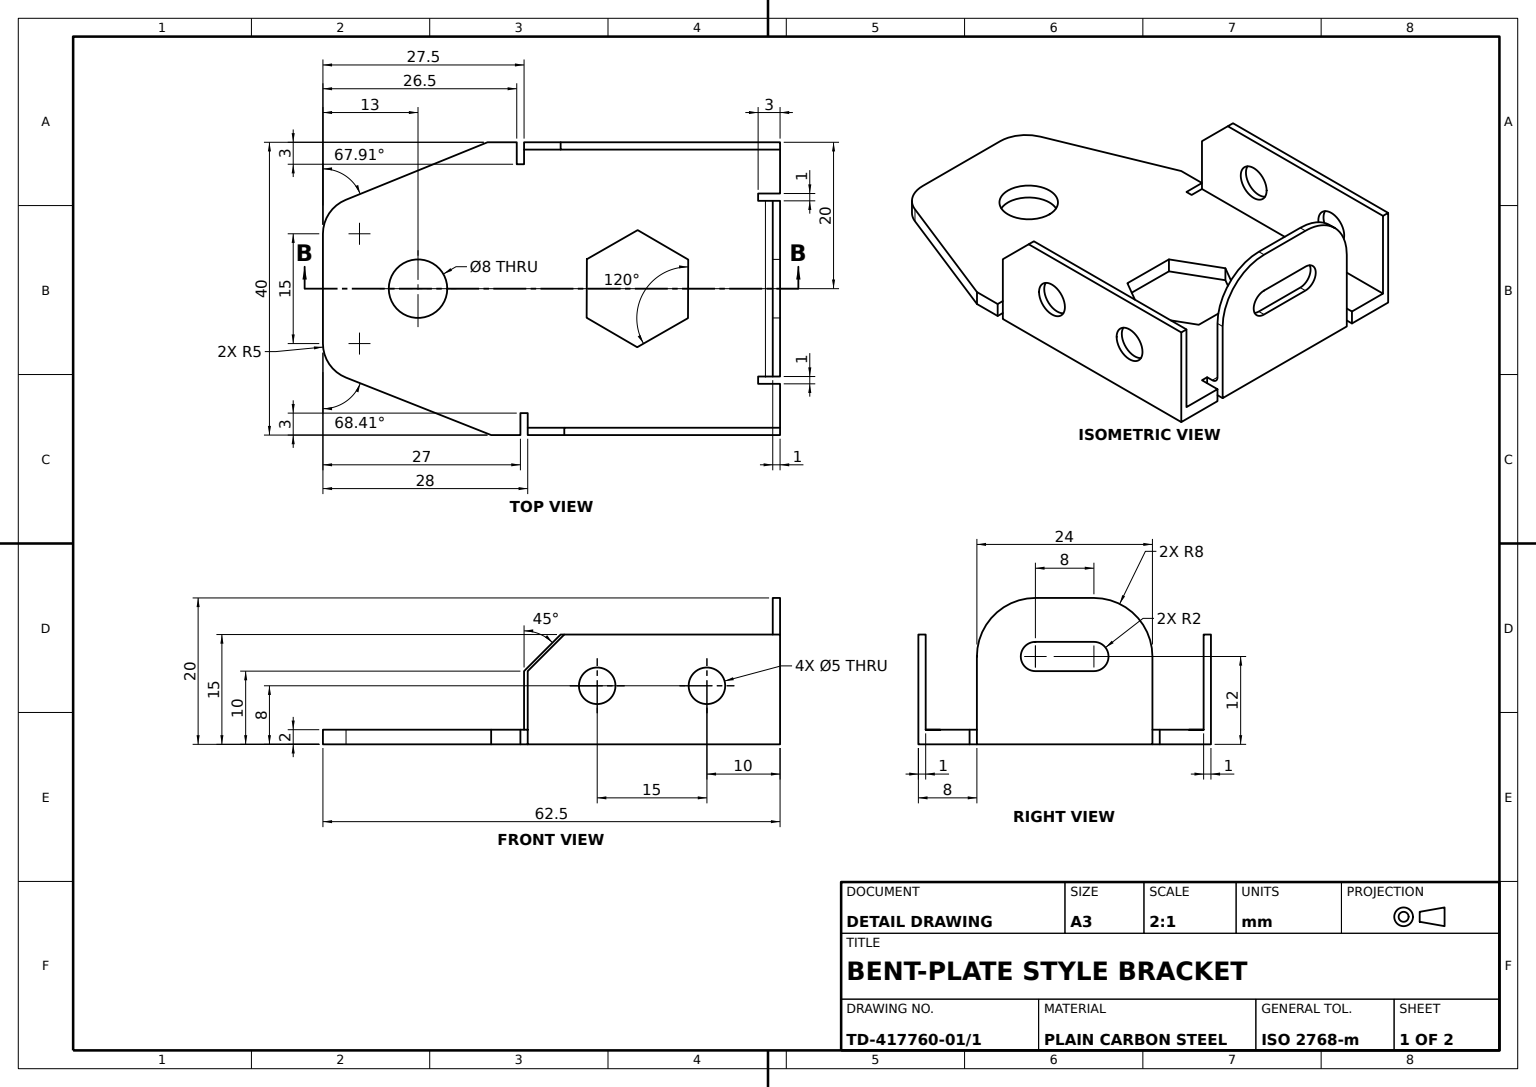
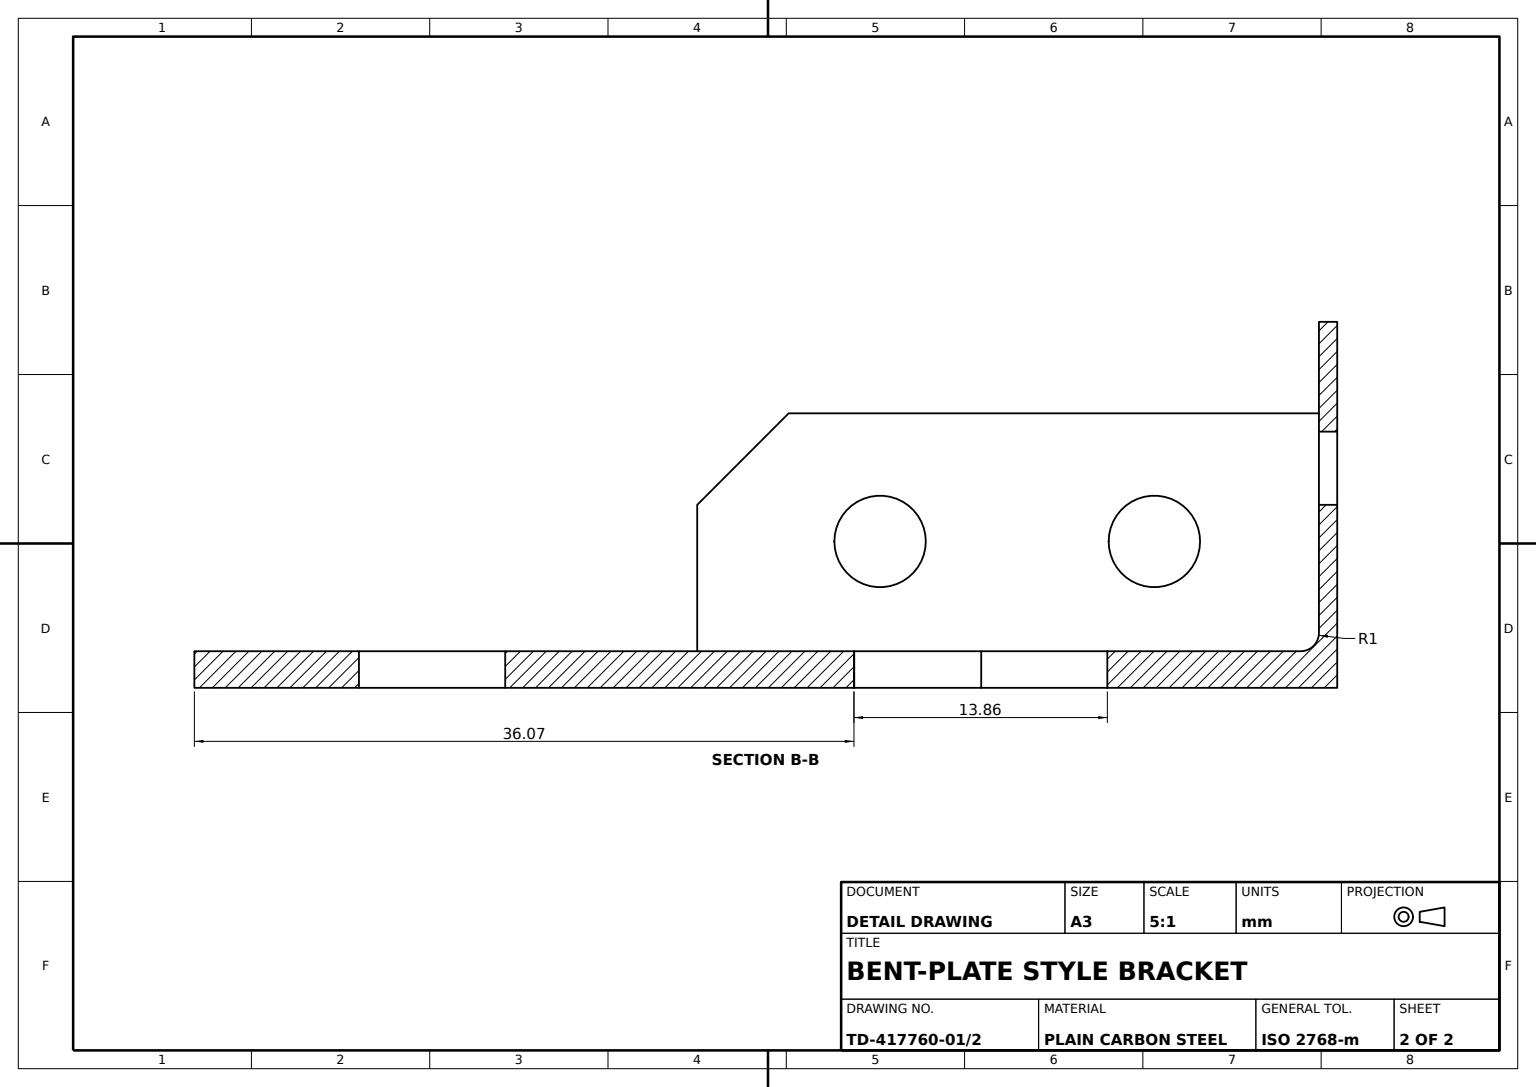
from build123d import *

# Parameters (mm, degrees)
BASE_PLATE_PROFILE_R        = 4
BASE_PLATE_PROFILE_W        = 1
BASE_PLATE_PROFILE_H        = 35
BASE_PLATE_PROFILE_W_2      = 24
BASE_PLATE_PROFILE_H_2      = 1
BASE_PLATE_PROFILE_H_3      = 34.5
BASE_PLATE_2MM_DEPTH        = 2
TAB_SEAT_RECESS_SKETCH_W    = 24
TAB_SEAT_RECESS_SKETCH_H    = 2
TAB_SEAT_RECESS_0_5MM_DEPTH = 0.5
SIDE_FLANGES_SKETCH_W       = 34.5
SIDE_FLANGES_SKETCH_H       = 2
SIDE_FLANGES_DEPTH          = 1
FLANGE_EXTENSION_DEPTH      = 1
REAR_TAB_SKETCH_W           = 24
REAR_TAB_SKETCH_H           = 20
REAR_TAB_24X20_DEPTH        = 1
REAR_TAB_CORNER_ROUND_R8_R  = 8
TAB_SLOT_DEPTH              = 2
TAB_ROOT_FILLET_R1_R        = 1
FLANGE_CROSS_HOLES_SKETCH_R = 2.5
FLANGE_CROSS_HOLES_DEPTH    = 50


with BuildPart() as part:
    # Base Plate Profile → Base Plate 2mm (new body)
    # profile 1 of 4: a face of its own
    with BuildSketch(Plane(origin=(0, 0, 0), x_dir=(1, 0, 0), z_dir=(0, 1, 0))):
        with BuildLine():
            Line((-13, 0), (-19, 0))
            Line((-19, 0), (-19, -35))
            Line((-19, -35), (-17, -35))
            Line((-17, -35), (-17, -36))
            Line((-17, -36), (-20, -36))
            Line((-20, -36), (-20, -40))
            Line((-20, -40), (-12.132851477, -59.380608198))
            ThreePointArc((-12.132851477, -59.380608198), (-10.292575783, -61.647471578), (-7.5, -62.5))
            Line((-7.5, -62.5), (7.5, -62.5))
            ThreePointArc((7.5, -62.5), (10.310807979, -61.63513706), (12.149230497, -59.339743401))
            Line((12.149230497, -59.339743401), (20, -39.5))
            Line((20, -39.5), (20, -35.5))
            Line((20, -35.5), (17, -35.5))
            Line((17, -35.5), (17, -34.5))
            Line((17, -34.5), (19, -34.5))
            Line((19, -34.5), (19, 0))
            Line((19, 0), (13, 0))
            Line((13, 0), (13, -3))
            Line((13, -3), (12, -3))
            Line((12, -3), (12, -0.5))
            Line((12, -0.5), (-12, -0.5))
            Line((-12, -0.5), (-12, -3))
            Line((-12, -3), (-13, -3))
            Line((-13, -3), (-13, 0))
        make_face()
        with Locations(Location((0, -49.5, 0), (0, 0, 270))):
            Circle(BASE_PLATE_PROFILE_R, mode=Mode.SUBTRACT)
        Polygon((8, -19.530894994), (3.97324415, -26.443650727), (-4.02675585, -26.412755733), (-8, -19.469105006), (-3.97324415, -12.556349273), (4.02675585, -12.587244267), align=None, mode=Mode.SUBTRACT)
    # profile 2 of 4: a face of its own
    with BuildSketch(Plane(origin=(0, 0, 0), x_dir=(1, 0, 0), z_dir=(0, 1, 0))):
        with Locations((-19.5, -17.5)):
            Rectangle(BASE_PLATE_PROFILE_W, BASE_PLATE_PROFILE_H)
    # profile 3 of 4: a face of its own
    with BuildSketch(Plane(origin=(0, 0, 0), x_dir=(1, 0, 0), z_dir=(0, 1, 0))):
        Rectangle(BASE_PLATE_PROFILE_W_2, BASE_PLATE_PROFILE_H_2)
    # profile 4 of 4: a face of its own
    with BuildSketch(Plane(origin=(0, 0, 0), x_dir=(1, 0, 0), z_dir=(0, 1, 0))):
        with Locations((19.5, -17.25)):
            Rectangle(BASE_PLATE_PROFILE_W, BASE_PLATE_PROFILE_H_3)
    extrude(amount=BASE_PLATE_2MM_DEPTH)

    # Tab Seat Recess Sketch → Tab Seat Recess 0.5mm (cut)
    with BuildSketch(Plane(origin=(0, 0, -0.5), x_dir=(-1, 0, 0), z_dir=(0, 0, -1))):
        with Locations((0, 1)):
            Rectangle(TAB_SEAT_RECESS_SKETCH_W, TAB_SEAT_RECESS_SKETCH_H)
    extrude(amount=-TAB_SEAT_RECESS_0_5MM_DEPTH, mode=Mode.SUBTRACT)

    # Side Flanges Sketch → Side Flanges (add)
    with BuildSketch(Plane(origin=(20, 0, 0), x_dir=(0, 0, -1), z_dir=(1, 0, 0))):
        Polygon((0, 15), (-29.5, 15), (-34.5, 10), (-34.5, 2), (0, 2), align=None)
        with Locations((-17.25, 1)):
            Rectangle(SIDE_FLANGES_SKETCH_W, SIDE_FLANGES_SKETCH_H)
    extrude(amount=-SIDE_FLANGES_DEPTH)

    # Flange Extension Sketch → Flange Extension (add)
    with BuildSketch(Plane.ZY.offset(20)):
        Polygon((0, 15), (0, 0), (35, 0), (35, 10), (30, 15), align=None)
    extrude(amount=-FLANGE_EXTENSION_DEPTH)

    # Rear Tab Sketch → Rear Tab 24x20 (add)
    with BuildSketch(Plane(origin=(0, 0, 0), x_dir=(-1, 0, 0), z_dir=(0, 0, -1))):
        with Locations((0, 10)):
            Rectangle(REAR_TAB_SKETCH_W, REAR_TAB_SKETCH_H)
    extrude(amount=-REAR_TAB_24X20_DEPTH)

    # Rear Tab Corner Round R8
    rear_tab_corner_round_r8_edges = [part.edges().sort_by_distance(p)[0] for p in [
        (12, 20, 0.5),
        (-12, 20, 0.5),
    ]]
    fillet(rear_tab_corner_round_r8_edges, radius=REAR_TAB_CORNER_ROUND_R8_R)

    # Tab Slot Sketch → Tab Slot (cut)
    with BuildSketch(Plane.XY.offset(1)):
        with BuildLine():
            Line((-3.998880062, 14), (3.998880062, 14))
            ThreePointArc((3.998880062, 14), (5.998880062, 12), (3.998880062, 10))
            Line((3.998880062, 10), (-3.998880062, 10))
            ThreePointArc((-3.998880062, 10), (-5.998880062, 12), (-3.998880062, 14))
        make_face()
    extrude(amount=-TAB_SLOT_DEPTH, mode=Mode.SUBTRACT)

    # Tab Root Fillet R1
    tab_root_fillet_r1_edges = [part.edges().sort_by_distance(p)[0] for p in [
        (0, 2, 1),
    ]]
    fillet(tab_root_fillet_r1_edges, radius=TAB_ROOT_FILLET_R1_R)

    # Flange Cross Holes Sketch → Flange Cross Holes (cut)
    with BuildSketch(Plane.ZY.offset(20)):
        with Locations((10, 8)):
            Circle(FLANGE_CROSS_HOLES_SKETCH_R)
        with Locations((25, 8)):
            Circle(FLANGE_CROSS_HOLES_SKETCH_R)
    extrude(amount=-FLANGE_CROSS_HOLES_DEPTH, mode=Mode.SUBTRACT)


solid = part.part
